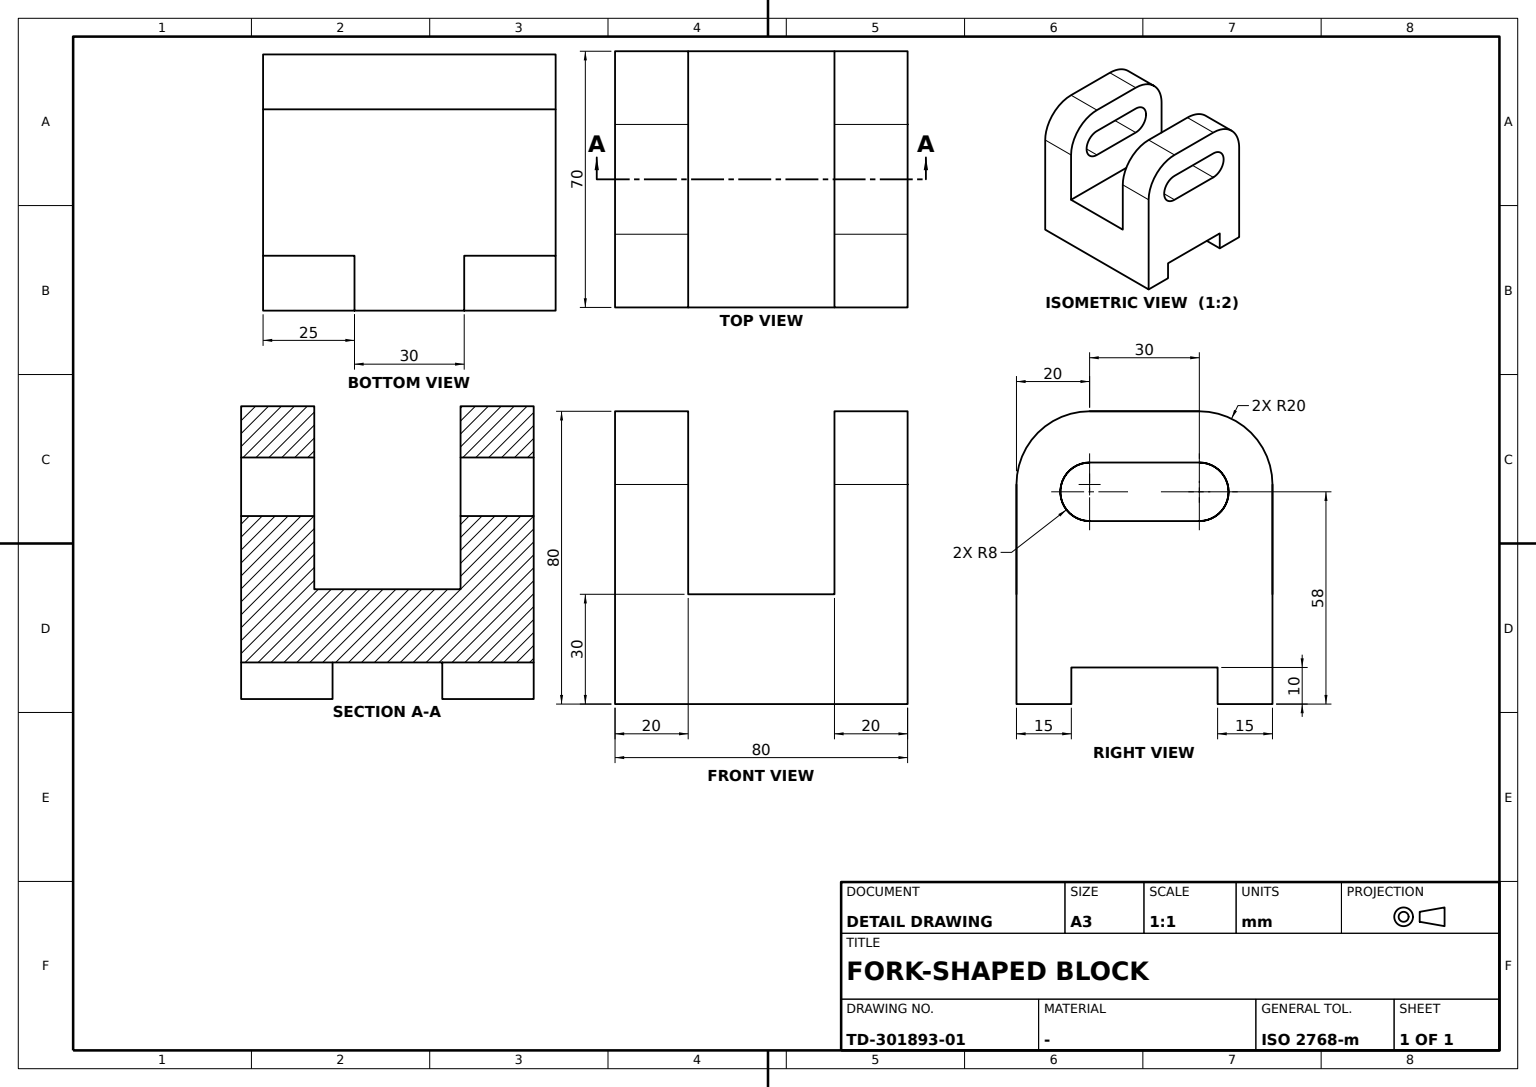
CATIA V5 part; units mm, degrees
sketch "Sketch1" plane through (0, 0, 0) normal (1, 0, 0) x (0, 1, 0)
  line L0 (-20, 0) -> (20, 0)
  line L1 (20, 0) -> (20, -10)
  line L2 (20, -10) -> (35, -10)
  point P0 (35, -10)
  line L3 (-20, 0) -> (-20, -10)
  point P1 (-20, -10)
  line L4 (-20, -10) -> (-35, -10)
  point P2 (-35, -10)
  line L5 (-35, -10) -> (-35, 70)
  line L6 (35, -10) -> (35, 70)
  line L7 (-35, 70) -> (35, 70)
  dimension "length L0" = 40
  dimension "length L1" = 10
  dimension "distance P0 y axis" = 35
  dimension "distance P2 y axis" = 35
  dimension "length L5" = 80
  constraint midpoint L0 origin
  constraint horizontal L0 x-axis
  constraint horizontal L2 x-axis
  constraint horizontal L4 x-axis
  constraint horizontal L7 x-axis
  constraint vertical L1 y-axis
  constraint vertical L3 y-axis
  constraint vertical L5 y-axis
  constraint vertical L6 y-axis
  constraint coincidence P1 L2
extrude "Pad1" add sketch "Sketch1" along normal mid plane 80
sketch "Sketch2" plane through (0, 35, 0) normal (0, 1, 0) x (-1, 0, 0)
  point P0 (0, 47.2308)
  line L0 (20, 74.4617) -> (20, 20)
  line L1 (20, 20) -> (-20, 20)
  line L2 (-20, 20) -> (-20, 74.4617)
  line L3 (-20, 74.4617) -> (20, 74.4617)
  line L4 (40, -10) -> (40, 70) construction
  line L5 (40, -10) -> (-40, -10) construction
  dimension "distance L0 L4" = 20
  dimension "distance L1 L5" = 30
  constraint coincidence P0 y-axis
  constraint vertical L0 y-axis
  constraint vertical L2 y-axis
  constraint horizontal L1 x-axis
  constraint horizontal L3 x-axis
  constraint equidistance L0 L2 P0
  constraint equidistance L1 L3 P0
extrude "Pocket1" cut sketch "Sketch2" against normal up to next
fillet "Fillet1" radius 20 1 edges at (30, 35, 70)
fillet "Fillet2" radius 20 1 edges at (-30, 35, 70)
fillet "Fillet3" radius 20 1 edges at (-30, -35, 70)
fillet "Fillet4" radius 20 1 edges at (30, -35, 70)
sketch "Sketch3" plane through (0, 35, 0) normal (0, 1, 0) x (-1, 0, 0)
  point P0 (0, -5)
  line L0 (15, 0) -> (15, -10)
  line L1 (15, -10) -> (-15, -10)
  line L2 (-15, -10) -> (-15, 0)
  line L3 (-15, 0) -> (15, 0)
  line L4 (40, -10) -> (-40, -10) construction
  dimension "length L0" = 10
  dimension "length L1" = 30
  constraint coincidence P0 y-axis
  constraint coincidence L1 L4
  constraint vertical L0 y-axis
  constraint vertical L2 y-axis
  constraint horizontal L1 x-axis
  constraint horizontal L3 x-axis
  constraint equidistance L0 L2 P0
  constraint equidistance L1 L3 P0
extrude "Pocket2" cut sketch "Sketch3" against normal up to next
sketch "Sketch4" plane through (40, 0, 0) normal (1, 0, 0) x (0, 1, 0)
  point P0 (0, 48)
  line L0 (15, 40) -> (-15, 40)
  line L1 (-15, 56) -> (15, 56)
  point P1 (15, 56)
  point P2 (15, 40)
  line L2 (35, 70) -> (-35, 70) construction
  arc A0 (15, 56) -> (15, 40) centre (15, 48) cw
  point P3 (15, 48)
  arc A1 (-15, 56) -> (-15, 40) centre (-15, 48) ccw
  dimension "distance P0 L2" = 22
  dimension "length L0" = 30
  dimension "distance P1 P2" = 16
  dimension "distance P3 y axis" = 15
  dimension "radius A0" = 8
  dimension "radius A1" = 8
  constraint coincidence P0 y-axis
  constraint horizontal L0 x-axis
  constraint horizontal L1 x-axis
  constraint equidistance L0 L1 P0
  constraint tangency A0 L0
  constraint tangency A1 L0
extrude "Pocket3" cut sketch "Sketch4" against normal through all
